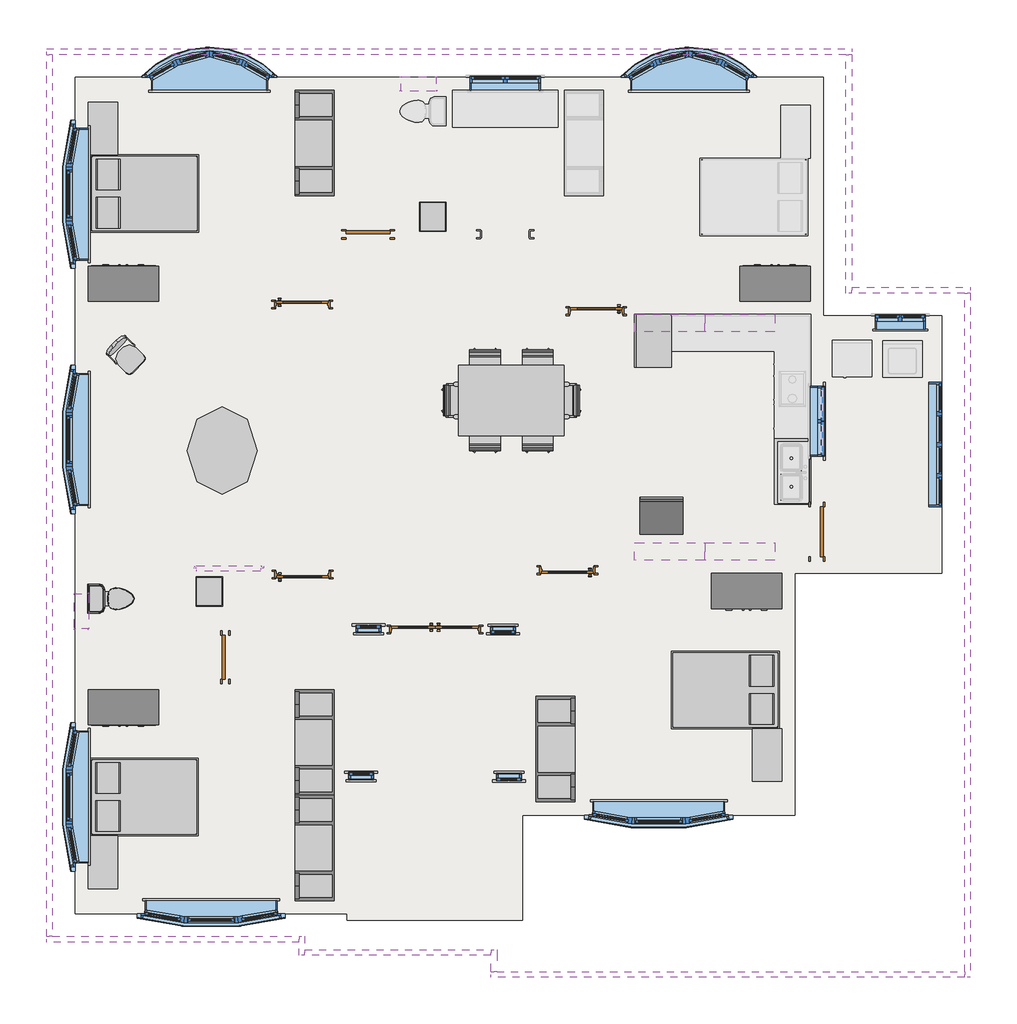
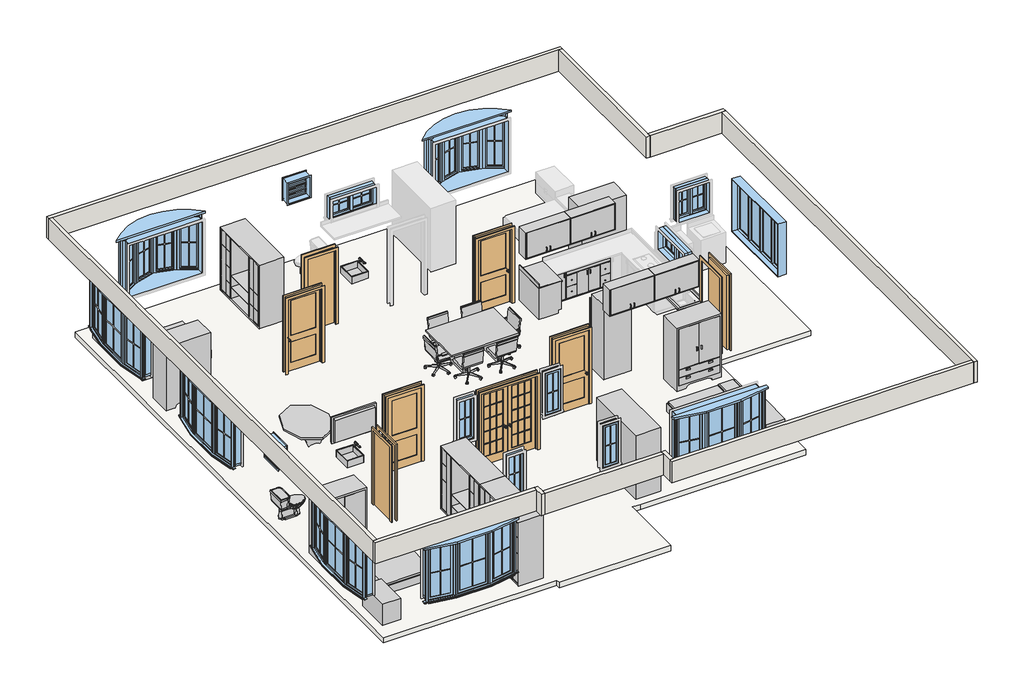
# One storey, part 1 of 2: 32 furniture elements, 17 windows, 10 walls, 8 doors, 3 flow terminals, 1 proxy, 1 slab.
# Revit data of these elements (continued)
# Element 59 (IfcWindow, "Window-Awning-Single : 17\" x 48\"") (continued)
#   Interior Wall Closure = 0' - 2 1/4"
#   Frame Extension = 0' - 0 1/4"
#   Exterior Wall Closure = 0' - 1 1/4"
#   Interior Trim Visibility = yes
#   Exterior Trim Visibility = yes
#   Phase Created = New Construction
#   Materials on its faces: "Wood - Stained", "Glass", "Clad - White"
# Element 60 (IfcWindow, "Window-Awning-Single : 17\" x 48\"")
#   Mark = "17"
#   Window Inset = 0' - 0"
#   Interior Wall Closure = 0' - 2 1/4"
#   Frame Extension = 0' - 0 1/4"
#   Exterior Wall Closure = 0' - 1 1/4"
#   Interior Trim Visibility = yes
#   Exterior Trim Visibility = yes
#   Phase Created = New Construction
#   Materials on its faces: "Wood - Stained", "Glass", "Clad - White"
# Element 61 (IfcWindow, "Window-Awning-Single : 17\" x 48\"")
#   Mark = "18"
#   Window Inset = 0' - 0"
#   Interior Wall Closure = 0' - 2 1/4"
#   Frame Extension = 0' - 0 1/4"
#   Exterior Wall Closure = 0' - 1 1/4"
#   Interior Trim Visibility = yes
#   Exterior Trim Visibility = yes
#   Phase Created = New Construction
#   Materials on its faces: "Wood - Stained", "Glass", "Clad - White"
# Element 62 (IfcWindow, "Window-Bay-Casement-10_Degree_Angle : 90\" x 60\" x 6\"")
#   Mark = "1"
#   Interior Trim Visibility = yes
#   Exterior Trim Visibility = yes
#   Phase Created = New Construction
#   Materials on its faces: "Clad - White", "Wood - Stained", "Glass"
# Element 63 (IfcWindow, "Window-Bay-Casement-10_Degree_Angle : 90\" x 60\" x 6\"")
#   Mark = "2"
#   Interior Trim Visibility = yes
#   Exterior Trim Visibility = yes
#   Phase Created = New Construction
#   Materials on its faces: "Clad - White", "Wood - Stained", "Glass"
# Element 64 (IfcWindow, "Window-Bay-Casement-10_Degree_Angle : 90\" x 60\" x 6\"")
#   Mark = "3"
#   Interior Trim Visibility = yes
#   Exterior Trim Visibility = yes
#   Phase Created = New Construction
#   Materials on its faces: "Clad - White", "Wood - Stained", "Glass"
# Element 65 (IfcWindow, "Window-Bay-Casement-10_Degree_Angle : 90\" x 60\" x 6\"")
#   Mark = "4"
#   Interior Trim Visibility = yes
#   Exterior Trim Visibility = yes
#   Phase Created = New Construction
#   Materials on its faces: "Clad - White", "Wood - Stained", "Glass"
# Element 66 (IfcWindow, "Window-Bay-Casement-10_Degree_Angle : 90\" x 60\" x 6\"")
#   Mark = "5"
#   Interior Trim Visibility = yes
#   Exterior Trim Visibility = yes
#   Phase Created = New Construction
#   Materials on its faces: "Clad - White", "Wood - Stained", "Glass"
# Element 67 (IfcWindow, "Window-Bow-Casement-15_Degree_Angle : 80\" x 60\"")
#   Mark = "7"
#   Interior Trim Visibility = yes
#   Exterior Trim Visibility = yes
#   Phase Created = New Construction
#   Materials on its faces: "Wood - Stained", "Clad - White", "Glass"
# Element 68 (IfcWindow, "Window-Bow-Casement-15_Degree_Angle : 80\" x 60\"")
#   Mark = "8"
#   Interior Trim Visibility = yes
#   Exterior Trim Visibility = yes
#   Phase Created = New Construction
#   Materials on its faces: "Wood - Stained", "Clad - White", "Glass"
# Element 69 (IfcWindow, "Window-Casement-Double : 34\" x 36\"")
#   Mark = "12"
#   Window Inset = 0' - 0"
#   Interior Wall Closure = 0' - 2 1/4"
#   Frame Extension = 0' - 0 1/4"
#   Exterior Wall Closure = 0' - 1 1/4"
#   Interior Trim Visibility = yes
#   Exterior Trim Visibility = yes
#   Phase Created = New Construction
#   Materials on its faces: "Wood - Stained", "Glass", "Clad - White"
# Element 70 (IfcWindow, "Window-Casement-Multi-Sash-Horizontal : 85\" x 60\"")
#   Mark = "11"
#   Window Inset = 0' - 0 5/8"
#   Frame Gap 3 = 0' - 1 83/128"
#   Frame Gap 2 = 0' - 0 5/8"
#   Phase Created = New Construction
#   Materials on its faces: "Metal - Aluminum", "Glass"
# Element 71 (IfcWindow, "Window-Louvers : 24\" x 24\"")
#   Mark = "13"
#   Blade Width = 1' - 10 1/2"
#   Phase Created = New Construction
#   Materials on its faces: "Birch"
# Element 72 (IfcWindow, "Window-Louvers : 24\" x 24\"")
#   Mark = "14"
#   Blade Width = 1' - 10 1/2"
#   Phase Created = New Construction
#   Materials on its faces: "Birch"
# Materials
#   "Metal - Paint Finish - Ivory,Glossy": colour RGB 247 247 239, transparency 0
#   "Cherry": class "Wood", colour RGB 226 177 128, transparency 0, Description = "Prunus Serotina", Cost = 0
#   "Aluminum": class "Metal", colour RGB 247 247 247, transparency 0, Description = "Aluminum 6061", Cost = 0
#   "Door - Panel": class "Wood", colour RGB 210 159 95, transparency 0, Cost = 0
#   "Door - Frame": colour RGB 118 70 51, transparency 0, Cost = 0
#   "Porcelain, Linen": class "Ceramic", colour RGB 249 239 230, transparency 0, Description = "Porcelain, linen", Cost = 0
#   "Laminate, Linen, Matte": class "Plastic", colour RGB 249 239 230, transparency 0, Description = "Plastic Laminate - Linen, Matte", Cost = 0
#   "Cabinets - Handles": colour RGB 57 57 57, transparency 0
#   "Cabinets": colour RGB 249 249 249, transparency 0
#   "Birch": class "Wood", colour RGB 224 178 126, transparency 0, Description = "Betula Alleghaniensis", Cost = 0
#   "Linen, White": class "Textile", colour RGB 247 247 239, transparency 0, Description = "Linen, white", Cost = 0
#   "Metal - Steel": colour RGB 210 210 210, transparency 0
#   "Plastic - Black": colour RGB 0 0 0, transparency 0.7
#   "Textile - Slate Blue": colour RGB 98 102 118, transparency 0
#   "Linen, Beige": class "Textile", colour RGB 249 239 230, transparency 0, Description = "Linen, beige", Cost = 0
#   "Steel, Paint Finish, Dark Gray, Matte": class "Metal", colour RGB 0 0 0, transparency 0, Description = "Steel, paint finish, dark gray, matte", Cost = 0
#   "Wood - Cherry": colour RGB 151 75 0, transparency 0
#   "Plastic - Gray": colour RGB 134 134 134, transparency 0
#   "Wood - Mahogany": colour RGB 138 86 45, transparency 0
#   "Concrete, Cast-in-Place gray": class "Concrete", colour RGB 192 192 192, transparency 0, Description = "Cast-in-place concrete", Cost = 0
#   "Wood - Stained": class "Wood", colour RGB 224 178 126, transparency 0, Cost = 0
#   "Glass": class "Glass", colour RGB 0 128 192, transparency 0.75, Description = "Soda Lime Glass", Cost = 0
#   "Clad - White": class "Wood", colour RGB 242 242 238, transparency 0, Cost = 0
#   "Metal - Aluminum": class "Metal", colour RGB 247 247 247, transparency 0
#   "Metal - Chrome": colour RGB 17 17 17, transparency 0
#   "Counter Top": class "Wood", colour RGB 226 177 128, transparency 0
#   "Steel, Chrome Plated": class "Metal", colour RGB 17 17 17, transparency 0, Description = "Chromiuim plated steel", Cost = 0
#   "Glass - Clear, Grey": class "Glass", colour RGB 252 255 255, transparency 0.64
#   "Cabinet": colour RGB 204 122 2, transparency 0
